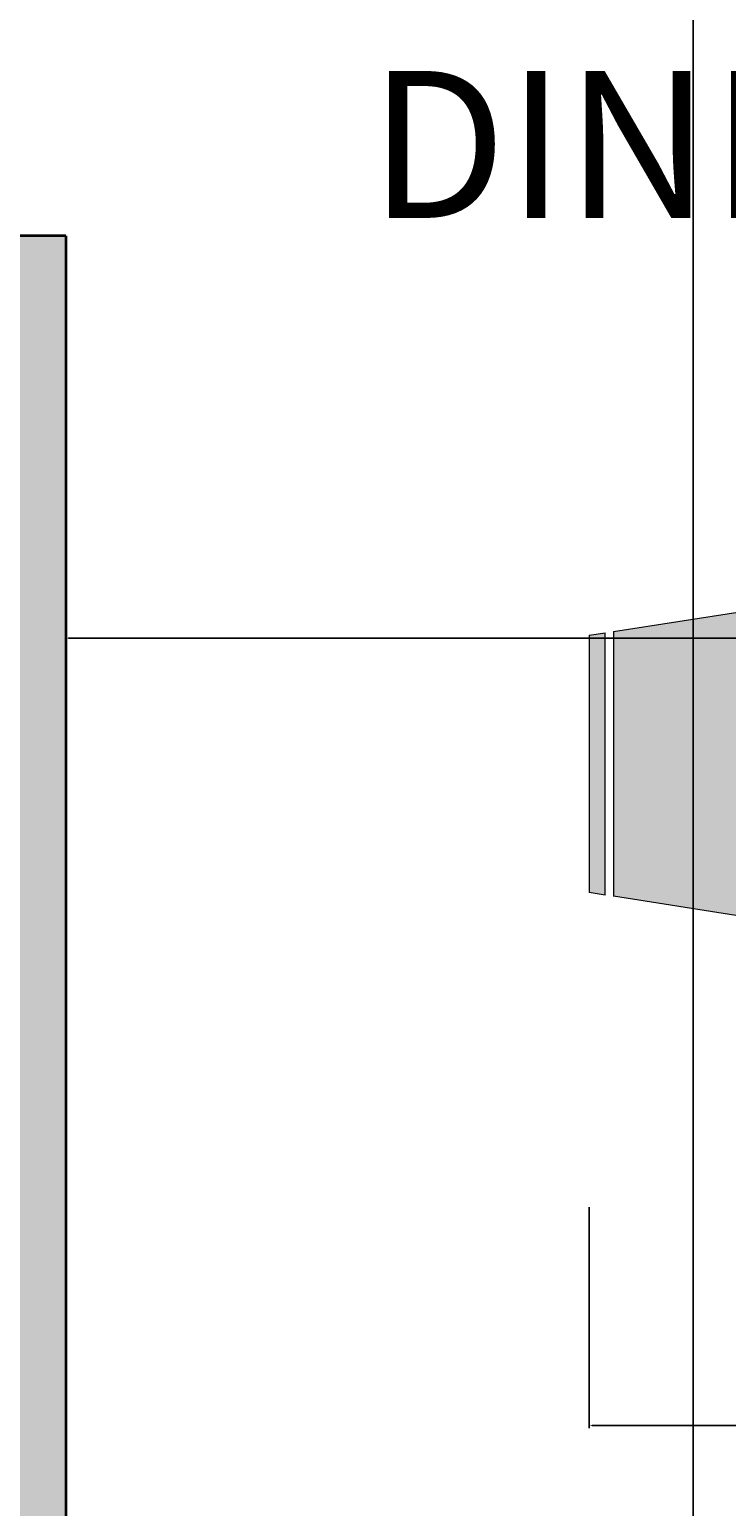
# Model space of a CAD drawing. Units: inches. Extents: x 1434 to 1845, y 1483 to 2014.
# Tile 4 of 11: x 1571 to 1615, y 1737 to 1829. Entities that reach past the tile are written whole.
import ezdxf

# ---------------------------------------------------------------- set-up
doc = ezdxf.new("R2010")
doc.units = ezdxf.units.IN
for name, color, linetype, lineweight in [('A-ANNO-DIMS', 2, 'Continuous', 18), ('A-AREA-IDEN', 7, 'Continuous', 25), ('A-FURN', 9, 'Continuous', 18), ('A-FURN-PATT', 9, 'Continuous', 13), ('A-WALL', 7, 'Continuous', 35), ('A-WALL-PATT', 8, 'Continuous', 13)]:
    doc.layers.add(name, color=color, linetype=linetype, lineweight=lineweight)
doc.styles.get("Standard").update_dxf_attribs({"font": 'arial.ttf'})
doc.dimstyles.get("Standard").update_dxf_attribs({"dimtxt": 0.18, "dimasz": 0.18, "dimexe": 0.18, "dimexo": 0.0625, "dimgap": 0.09, "dimtad": 0, "dimtih": 1, "dimtoh": 1, "dimdec": 4, "dimzin": 0, "dimdsep": 46, "dimtxsty": 'Standard', "dimcen": 0.09, "dimadec": 0, "dimazin": 0, "dimtfac": 1, "dimtdec": 4, "dimtofl": 0, "dimtmove": 0, "dimatfit": 3, "dimfxl": 1, "dimtolj": 1, "dimtzin": 0, "dimarcsym": 0})

# ---------------------------------------------------------------- blocks, each defined once
blk = doc.blocks.new('Dining Set - 36 x 72 in.')
for p, q in [((-22, 27.5), (-22.1562, 26.50042)), ((-22, 27.5), (-6, 27.5)), ((-5.8437, 26.49966), (-6, 27.5)), ((6, 27.5), (5.8438, 26.50042)), ((6, 27.5), (22, 27.5)), ((22.1563, 26.49966), (22, 27.5)), ((-22.2343, 26.00059), (-23.4847, 17.99762)), ((-22.2304, 26), (-5.7608, 26)), ((-5.8416, 26.5), (-22.1534, 26.5)), ((-4.5152, 17.99762), (-5.7655, 25.99926)), ((5.7657, 26.00059), (4.5153, 17.99762)), ((5.7696, 26), (22.2392, 26)), ((22.1584, 26.5), (5.8466, 26.5)), ((23.4848, 17.99762), (22.2345, 25.99926)), ((36, 18), (-36, 18)), ((-36, 18), (-36, -18)), ((36, -18), (36, 18)), ((-44.0006, 8.23428), (-35.9976, 9.48474)), ((44.0006, 8.23428), (35.9976, 9.48474)), ((-45.5, 8), (-44.5004, 8.15617)), ((-45.5, 8), (-45.5, -8)), ((-44.5, -8.15843), (-44.5, 8.15338)), ((-44, 8.23041), (-44, -8.23915)), ((44, 8.23041), (44, -8.23915)), ((44.5, -8.15843), (44.5, 8.15338)), ((45.5, 8), (44.5005, 8.15617)), ((45.5, 8), (45.5, -8)), ((-44.4997, -8.15631), (-45.5, -8)), ((-35.9976, -9.48476), (-43.9993, -8.2345)), ((35.9976, -9.48476), (43.9993, -8.2345)), ((44.4997, -8.15631), (45.5, -8)), ((-36, -18), (36, -18)), ((-22.2343, -26.0006), (-23.4847, -17.99762)), ((-4.5152, -17.99762), (-5.7655, -25.99928)), ((5.7657, -26.0006), (4.5153, -17.99762)), ((23.4848, -17.99762), (22.2345, -25.99928)), ((-22.2304, -26), (-5.7608, -26)), ((-22, -27.5), (-22.1562, -26.50044)), ((-5.8416, -26.5), (-22.1534, -26.5)), ((-5.8437, -26.49967), (-6, -27.5)), ((5.7696, -26), (22.2392, -26)), ((6, -27.5), (5.8438, -26.50044)), ((22.1584, -26.5), (5.8466, -26.5)), ((22.1563, -26.49967), (22, -27.5)), ((-22, -27.5), (-6, -27.5)), ((6, -27.5), (22, -27.5))]:
    blk.add_line(p, q)
for points in [[(-36, 15), (-31.1772, 14.97754), (-26.8079, 14.91406), (-22.8538, 14.81543), (-19.276, 14.6875), (-16.0362, 14.53613), (-13.0957, 14.36718), (-10.4159, 14.18652), (-7.9583, 14), (-5.6904, 13.81315), (-3.6035, 13.63021), (-1.6954, 13.45508), (0.0365, 13.29166), (1.5945, 13.14388), (2.9811, 13.01562), (4.1988, 12.9108), (5.25, 12.83333), (6.1393, 12.78613), (6.8802, 12.76823), (7.4883, 12.77767), (7.9792, 12.8125), (8.3685, 12.87077), (8.6719, 12.95052), (8.9049, 13.0498), (9.0833, 13.16666), (9.2205, 13.29899), (9.3216, 13.44401), (9.3895, 13.59879), (9.4271, 13.76041), (9.4373, 13.92594), (9.4232, 14.09245), (9.3875, 14.257), (9.3333, 14.41666), (9.2638, 14.56917), (9.1836, 14.71484), (9.0975, 14.85465), (9.0104, 14.98958), (8.9272, 15.1206), (8.8529, 15.2487), (8.7922, 15.37483), (8.75, 15.5), (8.7305, 15.62467), (8.7344, 15.74739), (8.7617, 15.86621), (8.8125, 15.97916), (8.8867, 16.08431), (8.9844, 16.17968), (9.1055, 16.26334), (9.25, 16.33333), (9.4189, 16.38802), (9.6172, 16.42708), (9.8506, 16.45052), (10.125, 16.45833), (10.4463, 16.45052), (10.8203, 16.42708), (11.2529, 16.38802), (11.75, 16.33333), (12.3184, 16.26318), (12.9694, 16.17838), (13.7151, 16.07991), (14.5677, 15.96875), (15.5395, 15.84586), (16.6426, 15.71224), (17.8893, 15.56884), (19.2917, 15.41666), (20.859, 15.25667), (22.5879, 15.08984), (24.4721, 14.91715), (26.5052, 14.73958), (28.6809, 14.5581), (30.9929, 14.3737), (33.4347, 14.18733), (36, 14)], [(-36, 10), (-28.9766, 10.14274), (-23.1725, 10.20442), (-18.4241, 10.19775), (-14.5677, 10.13541), (-11.4399, 10.03011), (-8.877, 9.89453), (-6.7154, 9.74137), (-4.7917, 9.58333), (-2.9698, 9.43082), (-1.2246, 9.28515), (0.4415, 9.14534), (2.026, 9.01041), (3.5266, 8.87939), (4.9408, 8.7513), (6.266, 8.62516), (7.5, 8.5), (8.6411, 8.37549), (9.6914, 8.2539), (10.6538, 8.13818), (11.5312, 8.03125), (12.3267, 7.93603), (13.043, 7.85547), (13.6831, 7.79248), (14.25, 7.75), (14.7471, 7.7303), (15.1797, 7.73307), (15.5537, 7.75732), (15.875, 7.80208), (16.1494, 7.86637), (16.3828, 7.94922), (16.5811, 8.04964), (16.75, 8.16666), (16.8944, 8.29915), (17.0143, 8.44531), (17.1089, 8.60319), (17.1771, 8.77083), (17.218, 8.94629), (17.2305, 9.1276), (17.2137, 9.31282), (17.1667, 9.5), (17.0895, 9.6875), (16.987, 9.875), (16.8649, 10.0625), (16.7292, 10.25), (16.5856, 10.4375), (16.4401, 10.625), (16.2985, 10.8125), (16.1667, 11), (16.05, 11.18733), (15.9518, 11.3737), (15.8752, 11.5581), (15.8229, 11.73958), (15.798, 11.91715), (15.8034, 12.08984), (15.842, 12.25667), (15.9167, 12.41666), (16.0295, 12.56836), (16.1784, 12.70833), (16.3605, 12.83268), (16.5729, 12.9375), (16.8127, 13.01888), (17.0768, 13.07291), (17.3625, 13.0957), (17.6667, 13.08333), (17.9894, 13.03312), (18.3418, 12.94726), (18.7382, 12.82918), (19.1927, 12.68229), (19.7195, 12.51001), (20.3327, 12.31575), (21.0465, 12.10294), (21.875, 11.875), (22.8357, 11.63354), (23.959, 11.37304), (25.2786, 11.08618), (26.8282, 10.76562), (28.6414, 10.40405), (30.752, 9.99414), (33.1936, 9.52856), (36, 9)], [(-36, 5.5), (-30.7157, 5.3348), (-26.069, 5.20963), (-21.9946, 5.11767), (-18.4271, 5.05208), (-15.3009, 5.00602), (-12.5508, 4.97265), (-10.1112, 4.94515), (-7.9167, 4.91666), (-5.909, 4.88167), (-4.0586, 4.83984), (-2.3429, 4.79215), (-0.7396, 4.73958), (0.7739, 4.6831), (2.22, 4.6237), (3.6213, 4.56233), (5, 4.5), (6.373, 4.43782), (7.7344, 4.3776), (9.0723, 4.32129), (10.375, 4.27083), (11.6309, 4.22819), (12.8281, 4.19531), (13.9551, 4.17415), (15, 4.16666), (15.954, 4.17448), (16.819, 4.19791), (17.6001, 4.23698), (18.3021, 4.29166), (18.9299, 4.36198), (19.4883, 4.44791), (19.9823, 4.54948), (20.4167, 4.66666), (20.7969, 4.79899), (21.1302, 4.94401), (21.4245, 5.09879), (21.6875, 5.26041), (21.9271, 5.42594), (22.1511, 5.59245), (22.3672, 5.757), (22.5834, 5.91666), (22.8065, 6.06868), (23.0404, 6.21093), (23.2879, 6.34147), (23.5521, 6.45833), (23.8358, 6.55957), (24.142, 6.64323), (24.4735, 6.70735), (24.8334, 6.75), (25.2235, 6.76969), (25.642, 6.76692), (26.0858, 6.74267), (26.5521, 6.69791), (27.0379, 6.63362), (27.5404, 6.55078), (28.0565, 6.45036), (28.5834, 6.33333), (29.1242, 6.19987), (29.7071, 6.04687), (30.3661, 5.87044), (31.1354, 5.66666), (32.0493, 5.43164), (33.142, 5.16146), (34.4475, 4.85221), (36, 4.5)], [(-36, -1), (-30.7915, -0.6591), (-26.0195, -0.38216), (-21.6519, -0.16284), (-17.6563, 0.00521), (-14.0005, 0.12833), (-10.6523, 0.21289), (-7.5796, 0.26522), (-4.75, 0.29166), (-2.134, 0.29793), (0.2878, 0.28711), (2.5317, 0.26163), (4.6146, 0.22396), (6.5529, 0.17651), (8.3633, 0.12174), (10.0623, 0.06209), (11.6667, 0), (13.1899, -0.06201), (14.6341, -0.1211), (15.9982, -0.17432), (17.2813, -0.21875), (18.4823, -0.25147), (19.6003, -0.26953), (20.6343, -0.27002), (21.5834, -0.25), (22.4481, -0.20768), (23.2357, -0.14584), (23.9549, -0.06836), (24.6146, 0.02083), (25.2235, 0.11784), (25.7904, 0.21875), (26.3241, 0.31966), (26.8334, 0.41666), (27.3265, 0.50618), (27.8099, 0.58593), (28.2894, 0.65397), (28.7709, 0.70833), (29.2601, 0.74707), (29.763, 0.76823), (30.2855, 0.76985), (30.8334, 0.75), (31.4088, 0.70784), (31.9994, 0.64713), (32.589, 0.57275), (33.1615, 0.48958), (33.7008, 0.4025), (34.1908, 0.3164), (34.6153, 0.23616), (34.9584, 0.16666), (35.2099, 0.11165), (35.3848, 0.07031), (35.504, 0.04069), (35.5886, 0.02083), (35.6594, 0.00879), (35.7377, 0.0026), (35.8442, 0.00032), (36, 0)], [(-36, -6.5), (-27.1843, -6.31267), (-20.084, -6.1263), (-14.469, -5.9419), (-10.1094, -5.76042), (-6.7752, -5.58285), (-4.2363, -5.41016), (-2.2629, -5.24333), (-0.625, -5.08334), (0.8708, -4.93099), (2.2715, -4.78646), (3.5872, -4.64974), (4.8281, -4.52084), (6.0046, -4.39974), (7.127, -4.28646), (8.2053, -4.18099), (9.25, -4.08334), (10.2705, -3.99382), (11.2734, -3.91407), (12.2647, -3.84603), (13.25, -3.79167), (14.2354, -3.75293), (15.2266, -3.73177), (16.2295, -3.73015), (17.25, -3.75), (18.2912, -3.79248), (19.3451, -3.85547), (20.4009, -3.93604), (21.4479, -4.03125), (22.4754, -4.13819), (23.4727, -4.25391), (24.4289, -4.37549), (25.3334, -4.5), (26.1785, -4.62492), (26.9694, -4.74935), (27.7145, -4.87281), (28.4219, -4.99479), (29.1, -5.11483), (29.7572, -5.23242), (30.4016, -5.34709), (31.0417, -5.45834), (31.6837, -5.56437), (32.3262, -5.65821), (32.9658, -5.73153), (33.599, -5.77604), (34.2224, -5.78345), (34.8327, -5.74545), (35.4264, -5.65373), (36, -5.5)], [(-36, -10), (-26.4022, -9.81299), (-18.4675, -9.62891), (-11.9839, -9.45069), (-6.7396, -9.28125), (-2.5226, -9.12354), (0.8789, -8.98047), (3.6769, -8.85498), (6.0833, -8.75), (8.2767, -8.66765), (10.3021, -8.60677), (12.1712, -8.56543), (13.8958, -8.54167), (15.4876, -8.53353), (16.9583, -8.53907), (18.3197, -8.55632), (19.5834, -8.58334), (20.7616, -8.61841), (21.8685, -8.66081), (22.9188, -8.71004), (23.9271, -8.76563), (24.9081, -8.82707), (25.8763, -8.89388), (26.8465, -8.96558), (27.8334, -9.04167), (28.8474, -9.12118), (29.8828, -9.20117), (30.93, -9.27824), (31.9792, -9.34896), (33.0205, -9.40991), (34.0443, -9.45768), (35.0407, -9.48885), (36, -9.5)], [(-36, -14.5), (-30.0881, -14.33513), (-25.0332, -14.21224), (-20.7312, -14.12647), (-17.0781, -14.07292), (-13.97, -14.04671), (-11.3027, -14.04297), (-8.9724, -14.05681), (-6.875, -14.08334), (-4.9224, -14.11833), (-3.0905, -14.16016), (-1.3709, -14.20785), (0.2448, -14.26042), (1.7647, -14.3169), (3.1973, -14.3763), (4.5507, -14.43767), (5.8333, -14.5), (7.0554, -14.5621), (8.235, -14.62175), (9.3922, -14.67652), (10.5469, -14.72396), (11.7192, -14.76164), (12.929, -14.78711), (14.1965, -14.79794), (15.5417, -14.79167), (16.9933, -14.76424), (18.6152, -14.70508), (20.4804, -14.60197), (22.6615, -14.44271), (25.2312, -14.21509), (28.2624, -13.9069), (31.8277, -13.50594), (36, -13)]]:
    blk.add_lwpolyline(points)
blk = doc.blocks.new('*D42')
at = {"layer": 'A-ANNO-DIMS', "color": 0, "lineweight": -2, "transparency": 16777216}
for p, q in [((1606.017, 1755.442), (1606.017, 1741.675)), ((1697.017, 1755.442), (1697.017, 1741.675)), ((1606.197, 1741.855), (1650.566, 1741.855)), ((1696.837, 1741.855), (1652.469, 1741.855))]:
    blk.add_line(p, q, dxfattribs=at)
at = {"layer": 'A-ANNO-DIMS', "color": 0, "transparency": 16777216}
for points in [[(1606.197, 1741.885), (1606.197, 1741.825), (1606.017, 1741.855)], [(1696.837, 1741.885), (1696.837, 1741.825), (1697.017, 1741.855)]]:
    blk.add_solid(points, dxfattribs=at)
at = {"layer": 'Defpoints', "color": 0, "transparency": 16777216}
for p in [(1606.017, 1755.505), (1697.017, 1755.505), (1697.017, 1741.855)]:
    blk.add_point(p, dxfattribs=at)
at = {"layer": 'A-ANNO-DIMS', "color": 0, "transparency": 16777216, "insert": (1651.517, 1741.855), "char_height": 0.18, "attachment_point": 5}
blk.add_mtext('\\A1;DINING SET 91', dxfattribs=at)
blk = doc.blocks.new('*D56')
at = {"layer": 'A-ANNO-DIMS', "color": 0, "lineweight": -2, "transparency": 16777216}
for p, q in [((1472.974, 1974.793), (1472.974, 1483.15)), ((1612.474, 1974.793), (1612.474, 1483.15)), ((1473.154, 1483.33), (1542.338, 1483.33)), ((1612.294, 1483.33), (1543.11, 1483.33))]:
    blk.add_line(p, q, dxfattribs=at)
at = {"layer": 'A-ANNO-DIMS', "color": 0, "transparency": 16777216}
for points in [[(1473.154, 1483.36), (1473.154, 1483.3), (1472.974, 1483.33)], [(1612.294, 1483.36), (1612.294, 1483.3), (1612.474, 1483.33)]]:
    blk.add_solid(points, dxfattribs=at)
at = {"layer": 'Defpoints', "color": 0, "transparency": 16777216}
for p in [(1472.974, 1974.855), (1612.474, 1974.855), (1612.474, 1483.33)]:
    blk.add_point(p, dxfattribs=at)
at = {"layer": 'A-ANNO-DIMS', "color": 0, "transparency": 16777216, "insert": (1542.724, 1483.33), "char_height": 0.18, "attachment_point": 5}
blk.add_mtext('\\A1;139.5', dxfattribs=at)
blk = doc.blocks.new('*D62')
at = {"layer": 'A-ANNO-DIMS', "color": 0, "lineweight": -2, "transparency": 16777216}
for p, q in [((1573.474, 1815.793), (1573.474, 1790.65)), ((1709.974, 1815.793), (1709.974, 1790.65)), ((1573.654, 1790.83), (1641.338, 1790.83)), ((1709.794, 1790.83), (1642.11, 1790.83))]:
    blk.add_line(p, q, dxfattribs=at)
at = {"layer": 'A-ANNO-DIMS', "color": 0, "transparency": 16777216}
for points in [[(1573.654, 1790.86), (1573.654, 1790.8), (1573.474, 1790.83)], [(1709.794, 1790.86), (1709.794, 1790.8), (1709.974, 1790.83)]]:
    blk.add_solid(points, dxfattribs=at)
at = {"layer": 'Defpoints', "color": 0, "transparency": 16777216}
for p in [(1573.474, 1815.855), (1709.974, 1815.855), (1573.474, 1790.83)]:
    blk.add_point(p, dxfattribs=at)
at = {"layer": 'A-ANNO-DIMS', "color": 0, "transparency": 16777216, "insert": (1641.724, 1790.83), "char_height": 0.18, "attachment_point": 5}
blk.add_mtext('\\A1;136.5', dxfattribs=at)

msp = doc.modelspace()

# ---------------------------------------------------------------- hatches: boundary and pattern name
at = {"layer": 'A-FURN-PATT'}
h = msp.add_hatch(color=256, dxfattribs=at)
h.dxf.hatch_style = 1
h.paths.add_polyline_path([(1673.6736, 1756.5049), (1657.3611, 1756.5049), (1657.5173, 1755.5049), (1673.5173, 1755.5049)])
h.paths.add_polyline_path([(1645.6736, 1756.5049), (1629.3611, 1756.5049), (1629.5173, 1755.5049), (1645.5173, 1755.5049)])
h.paths.add_polyline_path([(1697.0173, 1791.0049), (1696.0173, 1791.1611), (1696.0173, 1774.8486), (1697.0173, 1775.0049)])
h.paths.add_polyline_path([(1645.5173, 1810.5049), (1629.5173, 1810.5049), (1629.3611, 1809.5049), (1645.6736, 1809.5049)])
h.paths.add_polyline_path([(1673.5173, 1810.5049), (1657.5173, 1810.5049), (1657.3611, 1809.5049), (1673.6736, 1809.5049)])
h.paths.add_polyline_path([(1607.0173, 1791.1611), (1606.0173, 1791.0049), (1606.0173, 1775.0049), (1607.0173, 1774.8486)])
h = msp.add_hatch(color=256, dxfattribs=at)
h.dxf.hatch_style = 1
h.paths.add_polyline_path([(1673.7517, 1809.0049), (1657.2829, 1809.0049), (1656.033, 1801.0049), (1675.0018, 1801.0049)])
h.paths.add_polyline_path([(1645.7517, 1809.0049), (1629.2829, 1809.0049), (1628.033, 1801.0049), (1647.0018, 1801.0049)])
h.paths.add_polyline_path([(1647.0018, 1765.0049), (1628.033, 1765.0049), (1629.2829, 1757.0049), (1645.7517, 1757.0049)])
h.paths.add_polyline_path([(1615.5173, 1792.4892), (1607.5173, 1791.2392), (1607.5173, 1774.7705), (1615.5173, 1773.5205)])
h.paths.add_polyline_path([(1675.0018, 1765.0049), (1656.033, 1765.0049), (1657.2829, 1757.0049), (1673.7517, 1757.0049)])
h.paths.add_polyline_path([(1695.5173, 1791.2392), (1687.5173, 1792.4892), (1687.5173, 1773.5205), (1695.5173, 1774.7705)])
h.paths.add_polyline_path([(1491.9292, 1578.7679), (1493.2417, 1578.7679), (1493.1636, 1579.2679), (1476.6949, 1579.2679), (1476.6168, 1578.7679), (1477.9292, 1578.7679), (1475.9292, 1567.7679, -0.4833507), (1474.5739, 1565.6934), (1474.4292, 1564.7679, 0.4142136), (1475.4292, 1563.7679), (1484.9292, 1563.7679), (1494.4292, 1563.7679, 0.4142136), (1495.4292, 1564.7679), (1495.2846, 1565.6934, -0.4833518), (1493.9292, 1567.7679)])
h.paths.add_polyline_path([(1529.1236, 1578.8204), (1530.4361, 1578.8204), (1530.3579, 1579.3204), (1513.8892, 1579.3204), (1513.8111, 1578.8204), (1515.1236, 1578.8204), (1513.1236, 1567.8204, -0.4833507), (1511.7682, 1565.7459), (1511.6236, 1564.8204, 0.4142136), (1512.6236, 1563.8204), (1522.1236, 1563.8204), (1531.6236, 1563.8204, 0.4142136), (1532.6236, 1564.8204), (1532.4789, 1565.7459, -0.4833518), (1531.1236, 1567.8204)])
h.paths.add_polyline_path([(1531.8672, 1535.8802, -0.4833507), (1533.2226, 1537.9547), (1533.3672, 1538.8802, 0.4142136), (1532.3672, 1539.8802), (1522.8672, 1539.8802), (1513.3672, 1539.8802, 0.4142136), (1512.3672, 1538.8802), (1512.5118, 1537.9547, -0.4833518), (1513.8672, 1535.8802), (1515.8672, 1524.8802), (1514.5547, 1524.8802), (1514.6329, 1524.3802), (1531.1016, 1524.3802), (1531.1797, 1524.8802), (1529.8672, 1524.8802)])
h.paths.add_polyline_path([(1494.3799, 1536.0192, -0.4833507), (1495.7353, 1538.0938), (1495.8799, 1539.0192, 0.4142136), (1494.8799, 1540.0192), (1485.3799, 1540.0192), (1475.8799, 1540.0192, 0.4142136), (1474.8799, 1539.0192), (1475.0245, 1538.0938, -0.4833518), (1476.3799, 1536.0192), (1478.3799, 1525.0193), (1477.0674, 1525.0193), (1477.1456, 1524.5193), (1493.6143, 1524.5193), (1493.6924, 1525.0193), (1492.3799, 1525.0193)])
at = {"layer": 'A-WALL-PATT'}
h = msp.add_hatch(color=256, dxfattribs=at)
h.dxf.hatch_style = 1
h.paths.add_polyline_path([(1472.9742, 1730.3553), (1577.9742, 1730.3553), (1577.9742, 1734.8553), (1573.4742, 1734.8553), (1573.4742, 1815.8553), (1568.9742, 1815.8553), (1568.9742, 1734.8553), (1472.9742, 1734.8553), (1472.9742, 1770.1951), (1459.9742, 1770.1951), (1459.9742, 1782.1951), (1459.9742, 1818.1951), (1472.9742, 1818.1951), (1472.9742, 1854.8553), (1568.9742, 1854.8553), (1568.9742, 1851.8553), (1573.4742, 1851.8553), (1573.4742, 1854.8553), (1573.4742, 1859.3553), (1472.9742, 1859.3553), (1472.9742, 1899.9369), (1459.9742, 1899.9369), (1459.9742, 1911.9369), (1459.9742, 1947.9369), (1472.9742, 1947.9369), (1472.9742, 1974.8553), (1513.9785, 1974.8553), (1513.9785, 1987.8553), (1561.9785, 1987.8553), (1561.9785, 1974.8553), (1612.4742, 1974.8553), (1612.4742, 1859.3553), (1609.4742, 1859.3553), (1609.4742, 1854.8553), (1616.9742, 1854.8553), (1616.9742, 1910.3553), (1625.153, 1910.3553), (1625.153, 1914.8553), (1616.9742, 1914.8553), (1616.9742, 1988.3553), (1459.4742, 1988.3553), (1459.4742, 1508.3553), (1630.4742, 1508.3553), (1630.4742, 1517.3553), (1472.9742, 1517.3553), (1472.9742, 1586.3553), (1616.9742, 1586.3553), (1616.9742, 1583.3553), (1621.4742, 1583.3553), (1621.4742, 1586.3553), (1621.4742, 1734.8553), (1616.9742, 1734.8553), (1613.9742, 1734.8553), (1613.9742, 1730.3553), (1616.9742, 1730.3553), (1616.9742, 1590.8553), (1472.9742, 1590.8553), (1472.9742, 1635.7299), (1459.9742, 1635.7299), (1459.9742, 1647.7299), (1459.9742, 1683.7299), (1472.9742, 1683.7299)])
h.paths.add_polyline_path([(1819.4742, 1773.1667), (1810.4742, 1773.1667), (1810.4742, 1734.8553), (1714.4742, 1734.8553), (1714.4742, 1815.8553), (1709.9742, 1815.8553), (1709.9742, 1730.3553), (1745.9742, 1730.3553), (1745.9742, 1675.0848), (1753.4742, 1675.0848), (1753.4742, 1679.5848), (1750.4742, 1679.5848), (1750.4742, 1730.3553), (1810.4742, 1730.3553), (1810.4742, 1679.5848), (1792.4742, 1679.5848), (1792.4742, 1675.0848), (1810.4742, 1675.0848), (1810.4742, 1517.3553), (1775.1129, 1517.3553), (1775.1129, 1508.3553), (1819.4742, 1508.3553)])
h.paths.add_polyline_path([(1739.1129, 1517.3553), (1694.9742, 1517.3553), (1694.9742, 1730.3553), (1690.4742, 1730.3553), (1690.4742, 1517.3553), (1678.4742, 1517.3553), (1675.4742, 1517.3553), (1672.8212, 1517.3553), (1672.8212, 1508.3553), (1678.4742, 1508.3553), (1739.1129, 1508.3553)])
h.paths.add_polyline_path([(1735.6549, 1987.8553), (1783.6549, 1987.8553), (1783.6549, 1974.8553), (1810.4742, 1974.8553), (1810.4742, 1859.3553), (1709.9742, 1859.3553), (1709.9742, 1854.8553), (1709.9742, 1851.8553), (1714.4742, 1851.8553), (1714.4742, 1854.8553), (1810.4742, 1854.8553), (1810.4742, 1809.1667), (1819.4742, 1809.1667), (1819.4742, 1988.3553), (1666.4742, 1988.3553), (1666.4742, 1914.8553), (1661.1087, 1914.8553), (1661.1087, 1910.3553), (1666.4742, 1910.3553), (1666.4742, 1854.8553), (1673.9742, 1854.8553), (1673.9742, 1859.3553), (1670.9742, 1859.3553), (1670.9742, 1974.8553), (1735.6549, 1974.8553)])

# ---------------------------------------------------------------- linework, layer by layer
at = {"layer": 'A-WALL'}
for q in [(1568.9742, 1815.8553), (1573.4742, 1734.8553)]:
    msp.add_line((1573.4742, 1815.8553), q, dxfattribs=at)

# ---------------------------------------------------------------- block references
at = {"layer": 'A-FURN'}
msp.add_blockref('Dining Set - 36 x 72 in.', (1651.5173, 1783.0049), dxfattribs=at)

# ---------------------------------------------------------------- texts
at = {"layer": 'A-AREA-IDEN'}
msp.add_text('DINING / LIVING ', height=9.146682, dxfattribs=at).set_placement((1592.3026, 1816.9675))

# ---------------------------------------------------------------- dimensions: what is measured, and where the dimension line sits
at = {"layer": 'A-ANNO-DIMS'}
dim = msp.add_linear_dim(base=(1612.4742, 1483.3303), p1=(1472.9742, 1974.8553), p2=(1612.4742, 1974.8553), dimstyle='Standard', override={"dimdec": 1, "dimlfac": 1, "dimrnd": 0, "dimzin": 0, "dimdsep": 46, "dimlunit": 2}, dxfattribs=at)
dim.commit()
dim.dimension.update_dxf_attribs({"geometry": '*D56', "text_midpoint": (1542.7242, 1483.3303)})
dim = msp.add_linear_dim(base=(1573.4742, 1790.8303), p1=(1709.9742, 1815.8553), p2=(1573.4742, 1815.8553), angle=180, dimstyle='Standard', override={"dimdec": 1, "dimlfac": 1, "dimrnd": 0, "dimzin": 0, "dimdsep": 46, "dimlunit": 2}, dxfattribs=at)
dim.commit()
dim.dimension.update_dxf_attribs({"geometry": '*D62', "text_midpoint": (1641.7242, 1790.8303)})
dim = msp.add_linear_dim(base=(1697.0173, 1741.8549), p1=(1606.0173, 1755.5049), p2=(1697.0173, 1755.5049), text='DINING SET <>', dimstyle='Standard', override={"dimdec": 0, "dimlfac": 1, "dimrnd": 0, "dimzin": 0, "dimdsep": 46, "dimlunit": 2}, dxfattribs=at)
dim.commit()
dim.dimension.update_dxf_attribs({"geometry": '*D42', "text_midpoint": (1651.5173, 1741.8549)})

doc.saveas('drawing.dxf')
